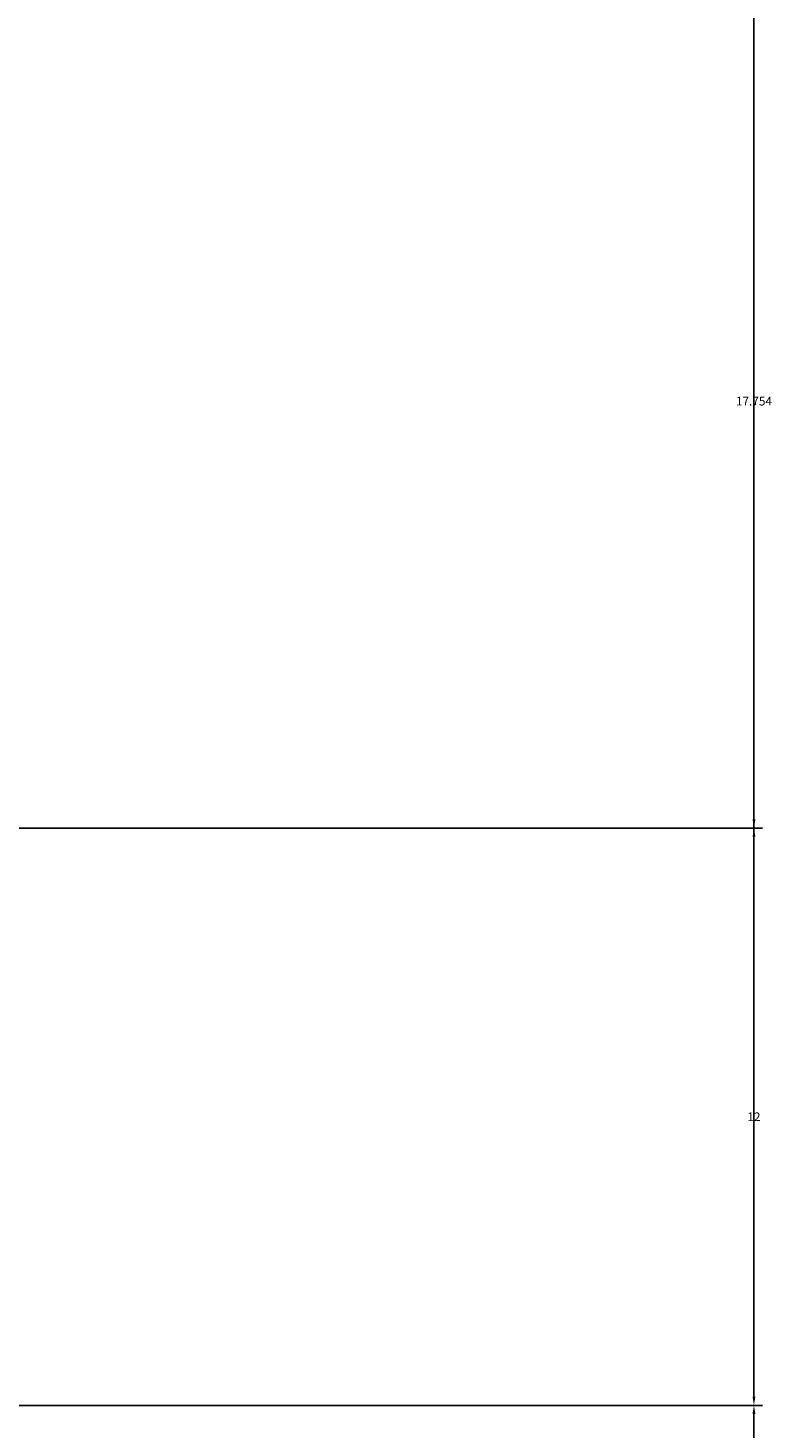
# Model space of a CAD drawing. Units: inches. Extents: x -6 to 289, y -8 to 323.
# Tile 99 of 107: x 273 to 289, y 247 to 276. Entities that reach past the tile are written whole.
import ezdxf

# ---------------------------------------------------------------- set-up
doc = ezdxf.new("R2010")
doc.units = ezdxf.units.IN
doc.header["$MEASUREMENT"] = 0
doc.layers.add('A-ANNO-DIMS', color=2, linetype='Continuous', lineweight=18)
doc.styles.get("Standard").update_dxf_attribs({"font": 'arial.ttf'})
doc.dimstyles.get("Standard").update_dxf_attribs({"dimtxt": 0.18, "dimasz": 0.18, "dimexe": 0.18, "dimexo": 0.0625, "dimgap": 0.09, "dimtad": 0, "dimtih": 1, "dimtoh": 1, "dimdec": 4, "dimzin": 0, "dimdsep": 46, "dimtxsty": 'Standard', "dimcen": 0.09, "dimadec": 0, "dimazin": 0, "dimtfac": 1, "dimtdec": 4, "dimtofl": 0, "dimtmove": 0, "dimatfit": 3, "dimfxl": 1, "dimtolj": 1, "dimtzin": 0, "dimarcsym": 0})

# ---------------------------------------------------------------- blocks, each defined once
blk = doc.blocks.new('*D26')
at = {"layer": 'A-ANNO-DIMS', "color": 0, "lineweight": -2, "transparency": 16777216}
for p, q in [((247.226, 247.289), (288.653, 247.289)), ((288.473, 247.109), (288.473, 237.153)), ((288.473, 226.834), (288.473, 236.789)), ((126.946, 226.654), (288.653, 226.654))]:
    blk.add_line(p, q, dxfattribs=at)
at = {"layer": 'A-ANNO-DIMS', "color": 0, "transparency": 16777216}
for points in [[(288.443, 247.109), (288.503, 247.109), (288.473, 247.289)], [(288.443, 226.834), (288.503, 226.834), (288.473, 226.654)]]:
    blk.add_solid(points, dxfattribs=at)
at = {"layer": 'Defpoints', "color": 0, "transparency": 16777216}
for p in [(247.164, 247.289), (288.473, 247.289), (126.883, 226.654)]:
    blk.add_point(p, dxfattribs=at)
at = {"layer": 'A-ANNO-DIMS', "color": 0, "transparency": 16777216, "insert": (288.473, 236.971), "char_height": 0.18, "attachment_point": 5}
blk.add_mtext('\\A1;20.635', dxfattribs=at)
blk = doc.blocks.new('*D27')
at = {"layer": 'A-ANNO-DIMS', "color": 0, "lineweight": -2, "transparency": 16777216}
for p, q in [((19.226, 307.289), (288.653, 307.289)), ((288.473, 307.109), (288.473, 277.471)), ((288.473, 247.469), (288.473, 277.107)), ((247.226, 247.289), (288.653, 247.289))]:
    blk.add_line(p, q, dxfattribs=at)
at = {"layer": 'A-ANNO-DIMS', "color": 0, "transparency": 16777216}
for points in [[(288.443, 307.109), (288.503, 307.109), (288.473, 307.289)], [(288.443, 247.469), (288.503, 247.469), (288.473, 247.289)]]:
    blk.add_solid(points, dxfattribs=at)
at = {"layer": 'Defpoints', "color": 0, "transparency": 16777216}
for p in [(19.164, 307.289), (288.473, 307.289), (247.164, 247.289)]:
    blk.add_point(p, dxfattribs=at)
at = {"layer": 'A-ANNO-DIMS', "color": 0, "transparency": 16777216, "insert": (288.473, 277.289), "char_height": 0.18, "attachment_point": 5}
blk.add_mtext('\\A1;60', dxfattribs=at)
blk = doc.blocks.new('*D113')
at = {"layer": 'A-ANNO-DIMS', "color": 0, "lineweight": -2, "transparency": 16777216}
for p, q in [((271.226, 259.289), (288.653, 259.289)), ((288.473, 259.109), (288.473, 253.469)), ((288.473, 247.469), (288.473, 253.108)), ((247.226, 247.289), (288.653, 247.289))]:
    blk.add_line(p, q, dxfattribs=at)
at = {"layer": 'A-ANNO-DIMS', "color": 0, "transparency": 16777216}
for points in [[(288.443, 259.109), (288.503, 259.109), (288.473, 259.289)], [(288.443, 247.469), (288.503, 247.469), (288.473, 247.289)]]:
    blk.add_solid(points, dxfattribs=at)
at = {"layer": 'Defpoints', "color": 0, "transparency": 16777216}
for p in [(271.164, 259.289), (288.473, 259.289), (247.164, 247.289)]:
    blk.add_point(p, dxfattribs=at)
at = {"layer": 'A-ANNO-DIMS', "color": 0, "transparency": 16777216, "insert": (288.473, 253.289), "char_height": 0.18, "attachment_point": 5}
blk.add_mtext('\\A1;12', dxfattribs=at)
blk = doc.blocks.new('*D114')
at = {"layer": 'A-ANNO-DIMS', "color": 0, "lineweight": -2, "transparency": 16777216}
for p, q in [((259.226, 277.043), (288.653, 277.043)), ((288.473, 276.863), (288.473, 268.348)), ((288.473, 259.469), (288.473, 267.984)), ((271.226, 259.289), (288.653, 259.289))]:
    blk.add_line(p, q, dxfattribs=at)
at = {"layer": 'A-ANNO-DIMS', "color": 0, "transparency": 16777216}
for points in [[(288.443, 276.863), (288.503, 276.863), (288.473, 277.043)], [(288.443, 259.469), (288.503, 259.469), (288.473, 259.289)]]:
    blk.add_solid(points, dxfattribs=at)
at = {"layer": 'Defpoints', "color": 0, "transparency": 16777216}
for p in [(259.164, 277.043), (288.473, 277.043), (271.164, 259.289)]:
    blk.add_point(p, dxfattribs=at)
at = {"layer": 'A-ANNO-DIMS', "color": 0, "transparency": 16777216, "insert": (288.473, 268.166), "char_height": 0.18, "attachment_point": 5}
blk.add_mtext('\\A1;17.754', dxfattribs=at)

msp = doc.modelspace()

# ---------------------------------------------------------------- dimensions: what is measured, and where the dimension line sits
at = {"layer": 'A-ANNO-DIMS'}
for base, p1, p2, override, picture, middle in [((288.4733, 307.2888), (247.1638, 247.2888), (19.1638, 307.2888), {"dimdec": 0, "dimlfac": 1, "dimrnd": 0, "dimzin": 0, "dimdsep": 46, "dimlunit": 2}, '*D27', (288.4733, 277.2888)), ((288.4733, 277.0427), (271.1638, 259.2888), (259.1638, 277.0427), {"dimdec": 3, "dimlfac": 1, "dimrnd": 0, "dimzin": 0, "dimdsep": 46, "dimlunit": 2}, '*D114', (288.4733, 268.1657)), ((288.4733, 259.2888), (247.1638, 247.2888), (271.1638, 259.2888), {"dimdec": 0, "dimlfac": 1, "dimrnd": 0, "dimzin": 0, "dimdsep": 46, "dimlunit": 2}, '*D113', (288.4733, 253.2888)), ((288.4733, 247.2888), (126.8835, 226.654), (247.1638, 247.2888), {"dimdec": 3, "dimlfac": 1, "dimrnd": 0, "dimzin": 0, "dimdsep": 46, "dimlunit": 2}, '*D26', (288.4733, 236.9714))]:
    dim = msp.add_linear_dim(base=base, p1=p1, p2=p2, angle=90, dimstyle='Standard', override=override, dxfattribs=at)
    dim.commit()
    dim.dimension.update_dxf_attribs({"geometry": picture, "text_midpoint": middle})

doc.saveas('drawing.dxf')
